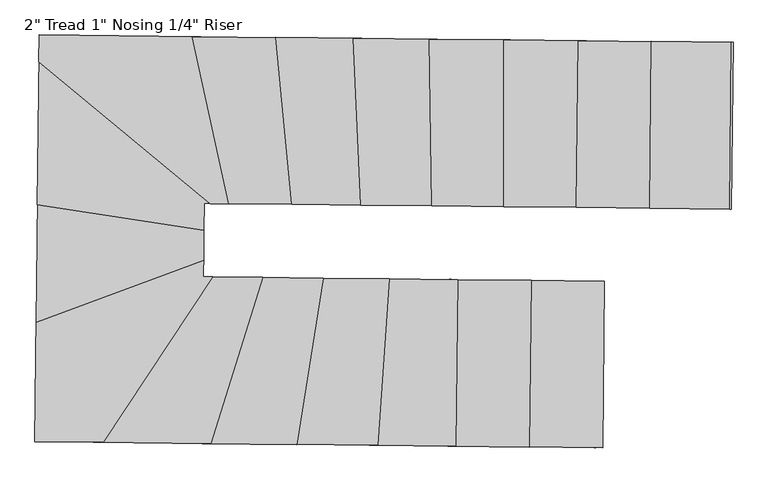
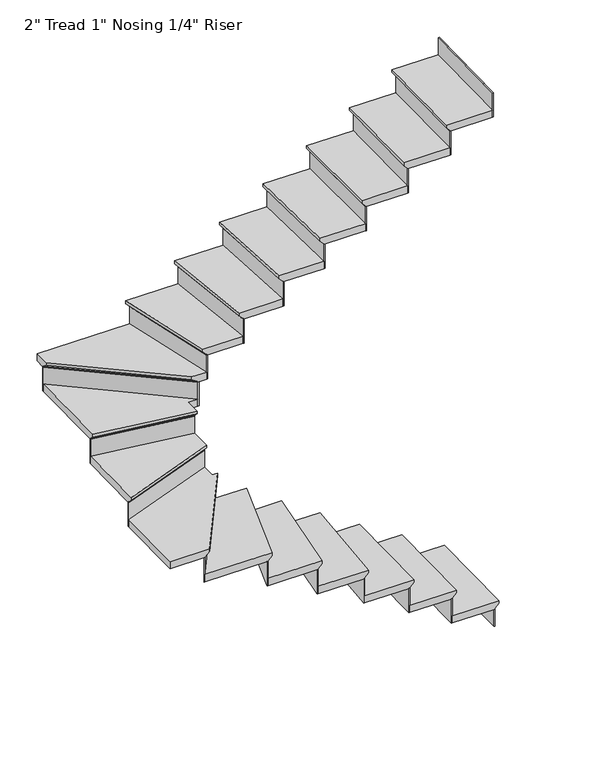
"""IFC4 building model written with IfcOpenShell, lengths in millimetres: stair flight geometry."""

from ifc_helpers import new_model, si_unit, origin, place, context, project, spatial, faceted_brep, source, transform, mapped, element, save


def stair_flight_bcee568d(model_context):
    return source(origin(), model_context, "Body", "Brep", [
        faceted_brep([(-1961.6349602, -4965.4067295, 150.2833333), (-1961.6349602, -4965.4067295, 169.3333333), (-1968.4523403, -5600.3701326, 169.3333333), (-1968.4523403, -5600.3701326, 150.2833333), (-1987.0334963, -4965.1340343, 124.8833333), (-1993.8508764, -5600.0974374, 124.8833333), (-2266.4173937, -4962.134387, 169.3333333), (-2273.2347738, -5597.0977902, 169.3333333), (-1993.8508764, -5600.0974374, 118.5333333), (-2273.2347738, -5597.0977902, 118.5333333), (-2266.4173937, -4962.134387, 118.5333333), (-1987.0334963, -4965.1340343, 118.5333333)], [[[0, 1, 2, 3]], [[4, 0, 3, 5]], [[2, 1, 6, 7]], [[8, 9, 10, 11]], [[2, 7, 9, 8, 5, 3]], [[8, 11, 4, 5]], [[6, 1, 0, 4, 11, 10]], [[7, 6, 10, 9]]]),
        faceted_brep([(-1987.0334963, -4965.1340343, 118.5333333), (-1987.0334963, -4965.1340343, 0.0), (-1993.3831304, -4965.0658605, 0.0), (-1993.3831304, -4965.0658605, 118.5333333), (-1993.8508764, -5600.0974374, 118.5333333), (-2000.2005104, -5600.0292636, 118.5333333), (-2000.2005104, -5600.0292636, 0.0), (-1993.8508764, -5600.0974374, 0.0)], [[[0, 1, 2, 3]], [[4, 5, 6, 7]], [[1, 0, 4, 7]], [[2, 1, 7, 6]], [[3, 2, 6, 5]], [[0, 3, 5, 4]]]),
        faceted_brep([(-2266.4173937, -4962.134387, 287.8666667), (-2266.4173937, -4962.134387, 118.5333333), (-2272.7670277, -4962.0662132, 118.5333333), (-2272.7670277, -4962.0662132, 287.8666667), (-2273.2347738, -5597.0977902, 287.8666667), (-2279.5844078, -5597.0296164, 287.8666667), (-2279.5844078, -5597.0296164, 118.5333333), (-2273.2347738, -5597.0977902, 118.5333333)], [[[0, 1, 2, 3]], [[4, 5, 6, 7]], [[1, 0, 4, 7]], [[2, 1, 7, 6]], [[3, 2, 6, 5]], [[0, 3, 5, 4]]]),
        faceted_brep([(-2247.8362377, -5597.3704854, 338.6666667), (-2241.0188576, -4962.4070822, 338.6666667), (-2545.8012911, -4959.1347398, 338.6666667), (-2552.6186712, -5594.0981429, 338.6666667), (-2273.2347738, -5597.0977902, 287.8666667), (-2552.6186712, -5594.0981429, 287.8666667), (-2545.8012911, -4959.1347398, 287.8666667), (-2266.4173937, -4962.134387, 287.8666667), (-2273.2347738, -5597.0977902, 294.2166667), (-2247.8362377, -5597.3704854, 319.6166667), (-2266.4173937, -4962.134387, 294.2166667), (-2241.0188576, -4962.4070822, 319.6166667)], [[[0, 1, 2, 3]], [[4, 5, 6, 7]], [[0, 3, 5, 4, 8, 9]], [[4, 7, 10, 8]], [[2, 1, 11, 10, 7, 6]], [[3, 2, 6, 5]], [[11, 1, 0, 9]], [[10, 11, 9, 8]]]),
        faceted_brep([(-2545.8012911, -4959.1347398, 457.2), (-2545.8012911, -4959.1347398, 287.8666667), (-2552.1509251, -4959.066566, 287.8666667), (-2552.1509251, -4959.066566, 457.2), (-2552.6186712, -5594.0981429, 457.2), (-2558.9683052, -5594.0299691, 457.2), (-2558.9683052, -5594.0299691, 287.8666667), (-2552.6186712, -5594.0981429, 287.8666667)], [[[0, 1, 2, 3]], [[4, 5, 6, 7]], [[1, 0, 4, 7]], [[2, 1, 7, 6]], [[3, 2, 6, 5]], [[0, 3, 5, 4]]]),
        faceted_brep([(-2527.2201351, -5594.3708381, 508.0), (-2520.402755, -4959.407435, 508.0), (-2806.7760852, -4956.3327447, 508.0), (-2850.4973934, -5590.8999232, 508.0), (-2552.6186712, -5594.0981429, 457.2), (-2850.4973934, -5590.8999232, 457.2), (-2806.7760852, -4956.3327447, 457.2), (-2545.8012911, -4959.1347398, 457.2), (-2552.6186712, -5594.0981429, 463.55), (-2527.2201351, -5594.3708381, 488.95), (-2545.8012911, -4959.1347398, 463.55), (-2520.402755, -4959.407435, 488.95)], [[[0, 1, 2, 3]], [[4, 5, 6, 7]], [[0, 3, 5, 4, 8, 9]], [[4, 7, 10, 8]], [[2, 1, 11, 10, 7, 6]], [[3, 2, 6, 5]], [[11, 1, 0, 9]], [[10, 11, 9, 8]]]),
        faceted_brep([(-2806.7760852, -4956.3327447, 626.5333333), (-2806.7760852, -4956.3327447, 457.2), (-2813.1364345, -4956.2644558, 457.2), (-2813.1364345, -4956.2644558, 626.5333333), (-2850.4973934, -5590.8999232, 626.5333333), (-2856.8577426, -5590.8316344, 626.5333333), (-2856.8577426, -5590.8316344, 457.2), (-2850.4973934, -5590.8999232, 457.2)], [[[0, 1, 2, 3]], [[4, 5, 6, 7]], [[1, 0, 4, 7]], [[2, 1, 7, 6]], [[3, 2, 6, 5]], [[0, 3, 5, 4]]]),
        faceted_brep([(-2825.0559965, -5591.1730786, 677.3333333), (-2781.3346883, -4956.6059001, 677.3333333), (-3058.0757112, -4953.6346284, 677.3333333), (-3158.4280189, -5587.5937798, 677.3333333), (-2850.4973934, -5590.8999232, 626.5333333), (-3158.4280189, -5587.5937798, 626.5333333), (-3058.0757112, -4953.6346284, 626.5333333), (-2806.7760852, -4956.3327447, 626.5333333), (-2850.4973934, -5590.8999232, 632.8833333), (-2825.0559965, -5591.1730786, 658.2833333), (-2806.7760852, -4956.3327447, 632.8833333), (-2781.3346883, -4956.6059001, 658.2833333)], [[[0, 1, 2, 3]], [[4, 5, 6, 7]], [[0, 3, 5, 4, 8, 9]], [[4, 7, 10, 8]], [[2, 1, 11, 10, 7, 6]], [[3, 2, 6, 5]], [[11, 1, 0, 9]], [[10, 11, 9, 8]]]),
        faceted_brep([(-3058.0757112, -4953.6346284, 795.8666667), (-3058.0757112, -4953.6346284, 626.5333333), (-3064.4938676, -4953.5657189, 626.5333333), (-3064.4938676, -4953.5657189, 795.8666667), (-3158.4280189, -5587.5937798, 795.8666667), (-3164.8461752, -5587.5248703, 795.8666667), (-3164.8461752, -5587.5248703, 626.5333333), (-3158.4280189, -5587.5937798, 626.5333333)], [[[0, 1, 2, 3]], [[4, 5, 6, 7]], [[1, 0, 4, 7]], [[2, 1, 7, 6]], [[3, 2, 6, 5]], [[0, 3, 5, 4]]]),
        faceted_brep([(-3132.7553936, -5587.8694178, 846.6666667), (-3032.4030859, -4953.9102664, 846.6666667), (-3289.3424431, -4951.1515984, 846.6666667), (-3487.6403792, -5584.0591417, 846.6666667), (-3158.4280189, -5587.5937798, 795.8666667), (-3487.6403792, -5584.0591417, 795.8666667), (-3289.3424431, -4951.1515984, 795.8666667), (-3058.0757112, -4953.6346284, 795.8666667), (-3158.4280189, -5587.5937798, 802.2166667), (-3132.7553936, -5587.8694178, 827.6166667), (-3058.0757112, -4953.6346284, 802.2166667), (-3032.4030859, -4953.9102664, 827.6166667)], [[[0, 1, 2, 3]], [[4, 5, 6, 7]], [[0, 3, 5, 4, 8, 9]], [[4, 7, 10, 8]], [[2, 1, 11, 10, 7, 6]], [[3, 2, 6, 5]], [[11, 1, 0, 9]], [[10, 11, 9, 8]]]),
        faceted_brep([(-3289.3424431, -4951.1515984, 965.2), (-3289.3424431, -4951.1515984, 795.8666667), (-3295.9745116, -4951.0803922, 795.8666667), (-3295.9745116, -4951.0803922, 965.2), (-3487.6403792, -5584.0591417, 965.2), (-3494.2724477, -5583.9879355, 965.2), (-3494.2724477, -5583.9879355, 795.8666667), (-3487.6403792, -5584.0591417, 795.8666667)], [[[0, 1, 2, 3]], [[4, 5, 6, 7]], [[1, 0, 4, 7]], [[2, 1, 7, 6]], [[3, 2, 6, 5]], [[0, 3, 5, 4]]]),
        faceted_brep([(-3461.1121052, -5584.3439665, 1016.0), (-3262.8141691, -4951.4364232, 1016.0), (-3484.2219113, -4949.0592457, 1016.0), (-3900.4163626, -5579.6273103, 1016.0), (-3487.6403792, -5584.0591417, 965.2), (-3900.4163626, -5579.6273103, 965.2), (-3484.2219113, -4949.0592457, 965.2), (-3289.3424431, -4951.1515984, 965.2), (-3487.6403792, -5584.0591417, 971.55), (-3461.1121052, -5584.3439665, 996.95), (-3289.3424431, -4951.1515984, 971.55), (-3262.8141691, -4951.4364232, 996.95)], [[[0, 1, 2, 3]], [[4, 5, 6, 7]], [[0, 3, 5, 4, 8, 9]], [[4, 7, 10, 8]], [[2, 1, 11, 10, 7, 6]], [[3, 2, 6, 5]], [[11, 1, 0, 9]], [[10, 11, 9, 8]]]),
        faceted_brep([(-3484.2219113, -4949.0592457, 1134.5333333), (-3484.2219113, -4949.0592457, 965.2), (-3491.7768309, -4948.9781311, 965.2), (-3491.7768309, -4948.9781311, 1134.5333333), (-3900.4163626, -5579.6273103, 1134.5333333), (-3907.9712823, -5579.5461958, 1134.5333333), (-3907.9712823, -5579.5461958, 965.2), (-3900.4163626, -5579.6273103, 965.2)], [[[0, 1, 2, 3]], [[4, 5, 6, 7]], [[1, 0, 4, 7]], [[2, 1, 7, 6]], [[3, 2, 6, 5]], [[0, 3, 5, 4]]]),
        faceted_brep([(-4125.8898698, -5095.6676694, 1185.3333333), (-4131.0593878, -5577.1509768, 1185.3333333), (-3870.196684, -5579.9517684, 1185.3333333), (-3454.0022327, -4949.3837038, 1185.3333333), (-3489.2786045, -4949.0049537, 1185.3333333), (-3488.312708, -4859.0423992, 1185.3333333), (-4131.0593878, -5577.1509768, 1134.5333333), (-4125.8898698, -5095.6676694, 1134.5333333), (-3488.312708, -4859.0423992, 1134.5333333), (-3489.2786045, -4949.0049537, 1134.5333333), (-3484.2219113, -4949.0592457, 1134.5333333), (-3900.4163626, -5579.6273103, 1134.5333333), (-3900.4163626, -5579.6273103, 1140.8833333), (-3870.196684, -5579.9517684, 1166.2833333), (-3484.2219113, -4949.0592457, 1140.8833333), (-3454.0022327, -4949.3837038, 1166.2833333)], [[[0, 1, 2, 3, 4, 5]], [[6, 7, 8, 9, 10, 11]], [[1, 0, 7, 6]], [[2, 1, 6, 11, 12, 13]], [[11, 10, 14, 12]], [[4, 3, 15, 14, 10, 9]], [[5, 4, 9, 8]], [[0, 5, 8, 7]], [[15, 3, 2, 13]], [[14, 15, 13, 12]]]),
        faceted_brep([(-3488.312708, -4859.0423992, 1303.8666667), (-3488.312708, -4859.0423992, 1134.5333333), (-3488.2396954, -4852.2420842, 1134.5333333), (-3488.2396954, -4852.2420842, 1303.8666667), (-4125.8898698, -5095.6676694, 1303.8666667), (-4125.8168572, -5088.8673543, 1303.8666667), (-4125.8168572, -5088.8673543, 1134.5333333), (-4125.8898698, -5095.6676694, 1134.5333333)], [[[0, 1, 2, 3]], [[4, 5, 6, 7]], [[1, 0, 4, 7]], [[2, 1, 7, 6]], [[3, 2, 6, 5]], [[0, 3, 5, 4]]]),
        faceted_brep([(-4126.1819202, -5122.8689296, 1354.6666667), (-3488.6047585, -4886.2436594, 1354.6666667), (-3487.1016265, -4746.243576, 1354.6666667), (-4121.0934321, -4648.9326558, 1354.6666667), (-4125.8898698, -5095.6676694, 1303.8666667), (-4121.0934321, -4648.9326558, 1303.8666667), (-3487.1016265, -4746.243576, 1303.8666667), (-3488.312708, -4859.0423992, 1303.8666667), (-4125.8898698, -5095.6676694, 1310.2166667), (-4126.1819202, -5122.8689296, 1335.6166667), (-3488.312708, -4859.0423992, 1310.2166667), (-3488.6047585, -4886.2436594, 1335.6166667)], [[[0, 1, 2, 3]], [[4, 5, 6, 7]], [[0, 3, 5, 4, 8, 9]], [[4, 7, 10, 8]], [[3, 2, 6, 5]], [[11, 1, 0, 9]], [[10, 11, 9, 8]], [[2, 1, 11, 10, 7, 6]]]),
        faceted_brep([(-3487.1016265, -4746.243576, 1473.2), (-3487.1016265, -4746.243576, 1303.8666667), (-3487.0327638, -4739.8297815, 1303.8666667), (-3487.0327638, -4739.8297815, 1473.2), (-4121.0934321, -4648.9326558, 1473.2), (-4121.0245695, -4642.5188612, 1473.2), (-4121.0245695, -4642.5188612, 1303.8666667), (-4121.0934321, -4648.9326558, 1303.8666667)], [[[0, 1, 2, 3]], [[4, 5, 6, 7]], [[1, 0, 4, 7]], [[2, 1, 7, 6]], [[3, 2, 6, 5]], [[0, 3, 5, 4]]]),
        faceted_brep([(-4121.3688828, -4674.587834, 1524.0), (-3487.3770772, -4771.8987542, 1524.0), (-3486.2789573, -4669.6210563, 1524.0), (-3423.6180491, -4670.2938246, 1524.0), (-4115.1699262, -4097.2237198, 1524.0), (-4121.0934321, -4648.9326558, 1473.2), (-4115.1699262, -4097.2237198, 1473.2), (-3423.6180491, -4670.2938246, 1473.2), (-3486.2789573, -4669.6210563, 1473.2), (-3487.1016265, -4746.243576, 1473.2), (-4121.0934321, -4648.9326558, 1479.55), (-4121.3688828, -4674.587834, 1504.95), (-3487.1016265, -4746.243576, 1479.55), (-3487.3770772, -4771.8987542, 1504.95)], [[[0, 1, 2, 3, 4]], [[5, 6, 7, 8, 9]], [[0, 4, 6, 5, 10, 11]], [[5, 9, 12, 10]], [[2, 1, 13, 12, 9, 8]], [[4, 3, 7, 6]], [[13, 1, 0, 11]], [[12, 13, 11, 10]], [[3, 2, 8, 7]]]),
        faceted_brep([(-3423.6180491, -4670.2938246, 1642.5333333), (-3423.6180491, -4670.2938246, 1473.2), (-3413.5354356, -4670.4020781, 1473.2), (-3413.5354356, -4670.4020781, 1642.5333333), (-4115.1699262, -4097.2237198, 1642.5333333), (-4115.0821626, -4089.0495147, 1642.5333333), (-4115.0821626, -4089.0495147, 1473.2), (-4115.1699262, -4097.2237198, 1473.2)], [[[0, 1, 2, 3]], [[4, 5, 6, 7]], [[1, 0, 4, 7]], [[2, 1, 7, 6]], [[3, 2, 6, 5]], [[0, 3, 5, 4]]]),
        faceted_brep([(-3506.4342514, -4034.368057, 1693.3333333), (-4114.4249804, -4027.8402731, 1693.3333333), (-4115.5209805, -4129.9205399, 1693.3333333), (-3463.9485035, -4669.8608106, 1693.3333333), (-3365.8789969, -4670.9137486, 1693.3333333), (-4114.4249804, -4027.8402731, 1642.5333333), (-3506.4342514, -4034.368057, 1642.5333333), (-3365.8789969, -4670.9137486, 1642.5333333), (-3423.6180491, -4670.2938246, 1642.5333333), (-4115.1699262, -4097.2237198, 1642.5333333), (-3423.6180491, -4670.2938246, 1648.8833333), (-4115.1699262, -4097.2237198, 1648.8833333), (-3463.9485035, -4669.8608106, 1674.2833333), (-4115.5209805, -4129.9205399, 1674.2833333)], [[[0, 1, 2, 3, 4]], [[5, 6, 7, 8, 9]], [[1, 0, 6, 5]], [[9, 8, 10, 11]], [[4, 3, 12, 10, 8, 7]], [[0, 4, 7, 6]], [[12, 3, 2, 13]], [[10, 12, 13, 11]], [[2, 1, 5, 9, 11, 13]]]),
        faceted_brep([(-3365.8789969, -4670.9137486, 1811.8666667), (-3365.8789969, -4670.9137486, 1642.5333333), (-3359.3605829, -4670.9837346, 1642.5333333), (-3359.3605829, -4670.9837346, 1811.8666667), (-3506.4342514, -4034.368057, 1811.8666667), (-3499.9158374, -4034.438043, 1811.8666667), (-3499.9158374, -4034.438043, 1642.5333333), (-3506.4342514, -4034.368057, 1642.5333333)], [[[0, 1, 2, 3]], [[4, 5, 6, 7]], [[1, 0, 4, 7]], [[2, 1, 7, 6]], [[3, 2, 6, 5]], [[0, 3, 5, 4]]]),
        faceted_brep([(-3532.5079076, -4034.0881133, 1862.6666667), (-3391.9526531, -4670.6338049, 1862.6666667), (-3127.2086135, -4673.4762691, 1862.6666667), (-3187.4049598, -4037.793363, 1862.6666667), (-3506.4342514, -4034.368057, 1811.8666667), (-3187.4049598, -4037.793363, 1811.8666667), (-3127.2086135, -4673.4762691, 1811.8666667), (-3365.8789969, -4670.9137486, 1811.8666667), (-3506.4342514, -4034.368057, 1818.2166667), (-3532.5079076, -4034.0881133, 1843.6166667), (-3365.8789969, -4670.9137486, 1818.2166667), (-3391.9526531, -4670.6338049, 1843.6166667)], [[[0, 1, 2, 3]], [[4, 5, 6, 7]], [[0, 3, 5, 4, 8, 9]], [[4, 7, 10, 8]], [[2, 1, 11, 10, 7, 6]], [[3, 2, 6, 5]], [[11, 1, 0, 9]], [[10, 11, 9, 8]]]),
        faceted_brep([(-3127.2086135, -4673.4762691, 1981.2), (-3127.2086135, -4673.4762691, 1811.8666667), (-3120.8237144, -4673.5448215, 1811.8666667), (-3120.8237144, -4673.5448215, 1981.2), (-3187.4049598, -4037.793363, 1981.2), (-3181.0200608, -4037.8619154, 1981.2), (-3181.0200608, -4037.8619154, 1811.8666667), (-3187.4049598, -4037.793363, 1811.8666667)], [[[0, 1, 2, 3]], [[4, 5, 6, 7]], [[1, 0, 4, 7]], [[2, 1, 7, 6]], [[3, 2, 6, 5]], [[0, 3, 5, 4]]]),
        faceted_brep([(-3212.9445562, -4037.5191533, 2032.0), (-3152.7482098, -4673.2020594, 2032.0), (-2863.8799111, -4676.3035373, 2032.0), (-2892.1704009, -4040.9631932, 2032.0), (-3187.4049598, -4037.793363, 1981.2), (-2892.1704009, -4040.9631932, 1981.2), (-2863.8799111, -4676.3035373, 1981.2), (-3127.2086135, -4673.4762691, 1981.2), (-3187.4049598, -4037.793363, 1987.55), (-3212.9445562, -4037.5191533, 2012.95), (-3127.2086135, -4673.4762691, 1987.55), (-3152.7482098, -4673.2020594, 2012.95)], [[[0, 1, 2, 3]], [[4, 5, 6, 7]], [[0, 3, 5, 4, 8, 9]], [[4, 7, 10, 8]], [[2, 1, 11, 10, 7, 6]], [[3, 2, 6, 5]], [[11, 1, 0, 9]], [[10, 11, 9, 8]]]),
        faceted_brep([(-2863.8799111, -4676.3035373, 2150.5333333), (-2863.8799111, -4676.3035373, 1981.2), (-2857.5205787, -4676.3718152, 1981.2), (-2857.5205787, -4676.3718152, 2150.5333333), (-2892.1704009, -4040.9631932, 2150.5333333), (-2885.8110685, -4041.0314712, 2150.5333333), (-2885.8110685, -4041.0314712, 1981.2), (-2892.1704009, -4040.9631932, 1981.2)], [[[0, 1, 2, 3]], [[4, 5, 6, 7]], [[1, 0, 4, 7]], [[2, 1, 7, 6]], [[3, 2, 6, 5]], [[0, 3, 5, 4]]]),
        faceted_brep([(-2917.6077305, -4040.6900815, 2201.3333333), (-2889.3172407, -4676.0304256, 2201.3333333), (-2593.0867697, -4679.2109486, 2201.3333333), (-2604.2529652, -4044.0544621, 2201.3333333), (-2892.1704009, -4040.9631932, 2150.5333333), (-2604.2529652, -4044.0544621, 2150.5333333), (-2593.0867697, -4679.2109486, 2150.5333333), (-2863.8799111, -4676.3035373, 2150.5333333), (-2892.1704009, -4040.9631932, 2156.8833333), (-2917.6077305, -4040.6900815, 2182.2833333), (-2863.8799111, -4676.3035373, 2156.8833333), (-2889.3172407, -4676.0304256, 2182.2833333)], [[[0, 1, 2, 3]], [[4, 5, 6, 7]], [[0, 3, 5, 4, 8, 9]], [[4, 7, 10, 8]], [[2, 1, 11, 10, 7, 6]], [[3, 2, 6, 5]], [[11, 1, 0, 9]], [[10, 11, 9, 8]]]),
        faceted_brep([(-2593.0867697, -4679.2109486, 2319.8666667), (-2593.0867697, -4679.2109486, 2150.5333333), (-2586.7345895, -4679.2791497, 2150.5333333), (-2586.7345895, -4679.2791497, 2319.8666667), (-2604.2529652, -4044.0544621, 2319.8666667), (-2597.900785, -4044.1226632, 2319.8666667), (-2597.900785, -4044.1226632, 2150.5333333), (-2604.2529652, -4044.0544621, 2150.5333333)], [[[0, 1, 2, 3]], [[4, 5, 6, 7]], [[1, 0, 4, 7]], [[2, 1, 7, 6]], [[3, 2, 6, 5]], [[0, 3, 5, 4]]]),
        faceted_brep([(-2629.661686, -4043.7816575, 2370.6666667), (-2618.4954904, -4678.9381441, 2370.6666667), (-2319.0528449, -4682.1531551, 2370.6666667), (-2319.536107, -4047.1113675, 2370.6666667), (-2604.2529652, -4044.0544621, 2319.8666667), (-2319.536107, -4047.1113675, 2319.8666667), (-2319.0528449, -4682.1531551, 2319.8666667), (-2593.0867697, -4679.2109486, 2319.8666667), (-2604.2529652, -4044.0544621, 2326.2166667), (-2629.661686, -4043.7816575, 2351.6166667), (-2593.0867697, -4679.2109486, 2326.2166667), (-2618.4954904, -4678.9381441, 2351.6166667)], [[[0, 1, 2, 3]], [[4, 5, 6, 7]], [[0, 3, 5, 4, 8, 9]], [[4, 7, 10, 8]], [[2, 1, 11, 10, 7, 6]], [[3, 2, 6, 5]], [[11, 1, 0, 9]], [[10, 11, 9, 8]]]),
        faceted_brep([(-2319.0528449, -4682.1531551, 2489.2), (-2319.0528449, -4682.1531551, 2319.8666667), (-2312.7027912, -4682.2213334, 2319.8666667), (-2312.7027912, -4682.2213334, 2489.2), (-2319.536107, -4047.1113675, 2489.2), (-2313.1860533, -4047.1795458, 2489.2), (-2313.1860533, -4047.1795458, 2319.8666667), (-2319.536107, -4047.1113675, 2319.8666667)], [[[0, 1, 2, 3]], [[4, 5, 6, 7]], [[1, 0, 4, 7]], [[2, 1, 7, 6]], [[3, 2, 6, 5]], [[0, 3, 5, 4]]]),
        faceted_brep([(-2344.9363219, -4046.8386542, 2540.0), (-2344.4530598, -4681.8804418, 2540.0), (-2043.3209474, -4685.113592, 2540.0), (-2036.5035673, -4050.1501889, 2540.0), (-2319.536107, -4047.1113675, 2489.2), (-2036.5035673, -4050.1501889, 2489.2), (-2043.3209474, -4685.113592, 2489.2), (-2319.0528449, -4682.1531551, 2489.2), (-2319.536107, -4047.1113675, 2495.55), (-2344.9363219, -4046.8386542, 2520.95), (-2319.0528449, -4682.1531551, 2495.55), (-2344.4530598, -4681.8804418, 2520.95)], [[[0, 1, 2, 3]], [[4, 5, 6, 7]], [[0, 3, 5, 4, 8, 9]], [[4, 7, 10, 8]], [[2, 1, 11, 10, 7, 6]], [[3, 2, 6, 5]], [[11, 1, 0, 9]], [[10, 11, 9, 8]]]),
        faceted_brep([(-2043.3209474, -4685.113592, 2658.5333333), (-2043.3209474, -4685.113592, 2489.2), (-2036.9713133, -4685.1817658, 2489.2), (-2036.9713133, -4685.1817658, 2658.5333333), (-2036.5035673, -4050.1501889, 2658.5333333), (-2030.1539332, -4050.2183627, 2658.5333333), (-2030.1539332, -4050.2183627, 2489.2), (-2036.5035673, -4050.1501889, 2489.2)], [[[0, 1, 2, 3]], [[4, 5, 6, 7]], [[1, 0, 4, 7]], [[2, 1, 7, 6]], [[3, 2, 6, 5]], [[0, 3, 5, 4]]]),
        faceted_brep([(-2061.9021034, -4049.8774937, 2709.3333333), (-2068.7194835, -4684.8408968, 2709.3333333), (-1763.93705, -4688.1132393, 2709.3333333), (-1757.1196699, -4053.1498361, 2709.3333333), (-2036.5035673, -4050.1501889, 2658.5333333), (-1757.1196699, -4053.1498361, 2658.5333333), (-1763.93705, -4688.1132393, 2658.5333333), (-2043.3209474, -4685.113592, 2658.5333333), (-2036.5035673, -4050.1501889, 2664.8833333), (-2061.9021034, -4049.8774937, 2690.2833333), (-2043.3209474, -4685.113592, 2664.8833333), (-2068.7194835, -4684.8408968, 2690.2833333)], [[[0, 1, 2, 3]], [[4, 5, 6, 7]], [[0, 3, 5, 4, 8, 9]], [[4, 7, 10, 8]], [[2, 1, 11, 10, 7, 6]], [[3, 2, 6, 5]], [[11, 1, 0, 9]], [[10, 11, 9, 8]]]),
        faceted_brep([(-1763.93705, -4688.1132393, 2827.8666667), (-1763.93705, -4688.1132393, 2658.5333333), (-1757.5874159, -4688.1814131, 2658.5333333), (-1757.5874159, -4688.1814131, 2827.8666667), (-1757.1196699, -4053.1498361, 2827.8666667), (-1750.7700359, -4053.2180099, 2827.8666667), (-1750.7700359, -4053.2180099, 2658.5333333), (-1757.1196699, -4053.1498361, 2658.5333333)], [[[0, 1, 2, 3]], [[4, 5, 6, 7]], [[1, 0, 4, 7]], [[2, 1, 7, 6]], [[3, 2, 6, 5]], [[0, 3, 5, 4]]]),
        faceted_brep([(-1484.5531526, -4691.1128865, 2997.2), (-1484.5531526, -4691.1128865, 2827.8666667), (-1478.2035186, -4691.1810603, 2827.8666667), (-1478.2035186, -4691.1810603, 2997.2), (-1477.7357725, -4056.1494834, 2997.2), (-1471.3861385, -4056.2176572, 2997.2), (-1471.3861385, -4056.2176572, 2827.8666667), (-1477.7357725, -4056.1494834, 2827.8666667)], [[[0, 1, 2, 3]], [[4, 5, 6, 7]], [[1, 0, 4, 7]], [[2, 1, 7, 6]], [[3, 2, 6, 5]], [[0, 3, 5, 4]]]),
        faceted_brep([(-1782.518206, -4052.8771409, 2878.6666667), (-1789.3355861, -4687.8405441, 2878.6666667), (-1484.5531526, -4691.1128865, 2878.6666667), (-1477.7357725, -4056.1494834, 2878.6666667), (-1757.1196699, -4053.1498361, 2827.8666667), (-1477.7357725, -4056.1494834, 2827.8666667), (-1484.5531526, -4691.1128865, 2827.8666667), (-1763.93705, -4688.1132393, 2827.8666667), (-1757.1196699, -4053.1498361, 2834.2166667), (-1782.518206, -4052.8771409, 2859.6166667), (-1763.93705, -4688.1132393, 2834.2166667), (-1789.3355861, -4687.8405441, 2859.6166667)], [[[0, 1, 2, 3]], [[4, 5, 6, 7]], [[0, 3, 5, 4, 8, 9]], [[4, 7, 10, 8]], [[2, 1, 11, 10, 7, 6]], [[3, 2, 6, 5]], [[11, 1, 0, 9]], [[10, 11, 9, 8]]]),
    ])


if __name__ == "__main__":
    model = new_model("IFC4")
    model_context = context("Model", 3, world=origin())
    ifc_project = project(units=[si_unit("LENGTHUNIT", "METRE", prefix="MILLI")], contexts=[model_context])
    site = spatial("IfcSite", under=ifc_project)
    building = spatial("IfcBuilding", under=site)
    placement = place(None, origin())
    stair_flight_shape = stair_flight_bcee568d(model_context)
    element("IfcStairFlight", 1, ObjectType="2\" Tread 1\" Nosing 1/4\" Riser", at=placement, inside=building, context=model_context, shape_type="MappedRepresentation", body=[
        mapped(stair_flight_shape, transform((0.0, 0.0, 0.0), x_axis=(1.0, 0.0, 0.0), y_axis=(0.0, 1.0, 0.0), z_axis=(0.0, 0.0, 1.0))),
    ])
    save(model, "model.ifc")
